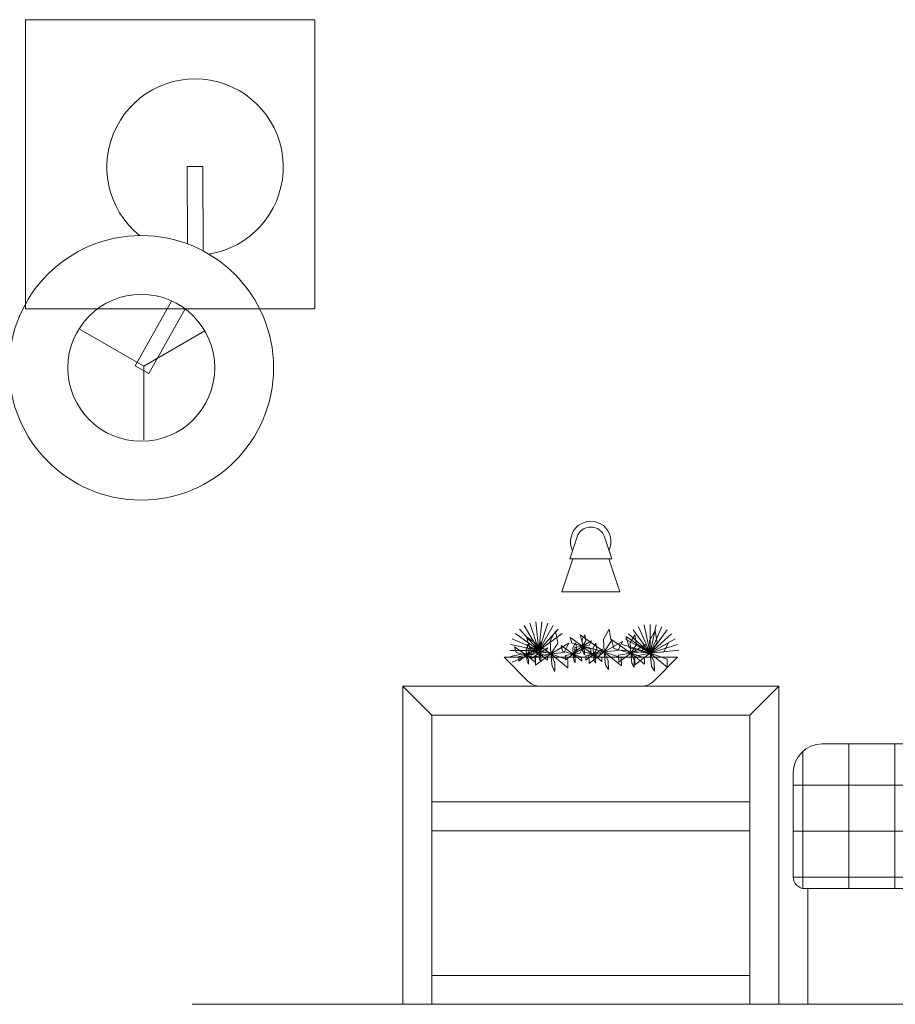
# Model space of a CAD drawing. Units: inches. Extents: x 1994 to 3075, y 3517 to 3950.
# Tile 26 of 58: x 1994.43113 to 1994.49073, y 3553.60329 to 3553.6703. Entities that reach past the tile are written whole.
import ezdxf

# ---------------------------------------------------------------- set-up
doc = ezdxf.new("R2010")
doc.units = ezdxf.units.IN
doc.layers.add('A-FURN-REFR', color=8, linetype='Continuous', lineweight=13)

msp = doc.modelspace()

# ---------------------------------------------------------------- linework, layer by layer
at = {"layer": 'A-FURN-REFR'}
for p, q in [((1994.431541370907, 3553.670297917026), (1994.431541370907, 3553.650612877656)), ((1994.451226410278, 3553.670297917026), (1994.431541370907, 3553.670297917026)), ((1994.451226410278, 3553.650612877656), (1994.451226410278, 3553.670297917026)), ((1994.442526696265, 3553.660297664388), (1994.443599002302, 3553.660302494364)), ((1994.442550361217, 3553.655043793864), (1994.442526696265, 3553.660297664388)), ((1994.443599002302, 3553.660302494364), (1994.443624860926, 3553.654561605301)), ((1994.438994690147, 3553.646750986684), (1994.441469284447, 3553.651146781573)), ((1994.431541370907, 3553.650612877656), (1994.451226410278, 3553.650612877656)), ((1994.442403711582, 3553.650620749735), (1994.439929117282, 3553.646224954846)), ((1994.439574063049, 3553.646711098967), (1994.43524393603, 3553.649211098967)), ((1994.439574063049, 3553.646711098967), (1994.443737547648, 3553.649114887921)), ((1994.439929117282, 3553.646224954846), (1994.438994690147, 3553.646750986684)), ((1994.439574063049, 3553.646711098967), (1994.439574063049, 3553.641711098967)), ((1994.468570884429, 3553.633608991265), (1994.469068334483, 3553.635101341428)), ((1994.471433271345, 3553.633608991265), (1994.470935821291, 3553.635101341428)), ((1994.46803357395, 3553.631374564225), (1994.468778382963, 3553.633608991265)), ((1994.468570884429, 3553.633608991264), (1994.471433271345, 3553.633608991265)), ((1994.471970581824, 3553.631374564225), (1994.471225772811, 3553.633608991265)), ((1994.46803357395, 3553.631374564225), (1994.471970581824, 3553.631374564225)), ((1994.465476211114, 3553.629074557141), (1994.466459409565, 3553.627369174909)), ((1994.466459409565, 3553.627369174909), (1994.465852265262, 3553.629241708899)), ((1994.46625485453, 3553.629327021937), (1994.466459409565, 3553.62736917491)), ((1994.466459409565, 3553.627369174909), (1994.466666383834, 3553.629326767666)), ((1994.46706886737, 3553.629240957197), (1994.466459409565, 3553.627369174909)), ((1994.466459409565, 3553.627369174909), (1994.467444714675, 3553.629073340861)), ((1994.473240709283, 3553.628979870546), (1994.474041371966, 3553.627181552716)), ((1994.474041371966, 3553.627181552716), (1994.473632096984, 3553.629107040119)), ((1994.474041371966, 3553.629150056654), (1994.474041371966, 3553.627181552716)), ((1994.474041371966, 3553.627181552716), (1994.474450646948, 3553.629107040119)), ((1994.474842034649, 3553.628979870546), (1994.474041371966, 3553.627181552716)), ((1994.466459409565, 3553.627369174909), (1994.464661586784, 3553.628170948567)), ((1994.464867571642, 3553.628527216263), (1994.466459409565, 3553.627369174909)), ((1994.466459409565, 3553.627369174909), (1994.465143127456, 3553.628832871995)), ((1994.46584606065, 3553.627531219063), (1994.465634292589, 3553.628302870623)), ((1994.465634292589, 3553.628302870623), (1994.467275044567, 3553.627153687641)), ((1994.467777499419, 3553.628831244294), (1994.466459409565, 3553.62736917491)), ((1994.466459409565, 3553.627369174909), (1994.468052677311, 3553.628525248281)), ((1994.467606987953, 3553.628694062704), (1994.467232384733, 3553.628020558311)), ((1994.467761039117, 3553.627872780074), (1994.467606987953, 3553.628694062704)), ((1994.468714541152, 3553.62786448459), (1994.468608657122, 3553.62825031037)), ((1994.468608657122, 3553.62825031037), (1994.469429033111, 3553.627675718879)), ((1994.469483494406, 3553.62765450469), (1994.469271726346, 3553.62842615625)), ((1994.469271726346, 3553.62842615625), (1994.470912478323, 3553.627276973268)), ((1994.469595004804, 3553.628445906411), (1994.469407703195, 3553.628109154214)), ((1994.469672030386, 3553.628035265095), (1994.469595004804, 3553.628445906411)), ((1994.471244421709, 3553.628817348331), (1994.47086981849, 3553.628143843938)), ((1994.471398472873, 3553.627996065702), (1994.471244421709, 3553.628817348331)), ((1994.472612388051, 3553.627559084138), (1994.47240061999, 3553.628330735697)), ((1994.47240061999, 3553.628330735697), (1994.474041371967, 3553.627181552715)), ((1994.472578488451, 3553.628498738949), (1994.474041371965, 3553.627181552716)), ((1994.472990738656, 3553.628432239769), (1994.47269105608, 3553.627893436255)), ((1994.474041371967, 3553.627181552716), (1994.472884314383, 3553.628774105855)), ((1994.473113979587, 3553.627775213666), (1994.472990738656, 3553.628432239769)), ((1994.474373315353, 3553.628721927778), (1994.473998712134, 3553.628048423386)), ((1994.474041371966, 3553.627181552716), (1994.475198429549, 3553.628774105855)), ((1994.475504255481, 3553.628498738949), (1994.474041371966, 3553.627181552716)), ((1994.474527366517, 3553.627900645149), (1994.474373315353, 3553.628721927778)), ((1994.464534175408, 3553.627779639515), (1994.466459409564, 3553.627369174909)), ((1994.464914215042, 3553.627238030449), (1994.464808331011, 3553.627623856228)), ((1994.464808331011, 3553.627623856228), (1994.465628707, 3553.627049264738)), ((1994.465794678693, 3553.627819452269), (1994.465607377083, 3553.627482700072)), ((1994.465753568113, 3553.627382157664), (1994.465647684083, 3553.627767983443)), ((1994.465647684083, 3553.627767983443), (1994.466468060071, 3553.627193391952)), ((1994.465871704275, 3553.627408810954), (1994.465794678693, 3553.627819452269)), ((1994.467275044567, 3553.627153687641), (1994.46584606065, 3553.627531219063)), ((1994.466634031764, 3553.627963579483), (1994.466446730155, 3553.627626827287)), ((1994.466446730155, 3553.627626827287), (1994.466468060071, 3553.627193391952)), ((1994.466468060071, 3553.627193391952), (1994.466711057347, 3553.627552938169)), ((1994.466468060071, 3553.627193391952), (1994.467088797114, 3553.627551474141)), ((1994.466711057347, 3553.627552938169), (1994.466634031764, 3553.627963579483)), ((1994.467088797114, 3553.627551474141), (1994.466930353947, 3553.62723953747)), ((1994.467232384733, 3553.628020558311), (1994.467275044567, 3553.627153687641)), ((1994.467275044567, 3553.627153687641), (1994.467761039117, 3553.627872780074)), ((1994.467275044567, 3553.627153687641), (1994.468516518652, 3553.627869852017)), ((1994.468085970577, 3553.627317511473), (1994.467980086547, 3553.627703337253)), ((1994.467980086547, 3553.627703337253), (1994.468800462536, 3553.627128745762)), ((1994.468516518652, 3553.627869852017), (1994.468199632319, 3553.627245978677)), ((1994.469429033111, 3553.627675718879), (1994.468714541152, 3553.62786448459)), ((1994.468966434229, 3553.627898933294), (1994.468779132619, 3553.627562181097)), ((1994.468779132619, 3553.627562181097), (1994.468800462536, 3553.627128745762)), ((1994.469429033111, 3553.627675718879), (1994.468909022243, 3553.627579942366)), ((1994.468909022243, 3553.627579942366), (1994.468913622717, 3553.627282713637)), ((1994.468913622717, 3553.627282713637), (1994.469429033111, 3553.627675718879)), ((1994.469043459811, 3553.627488291979), (1994.468966434229, 3553.627898933294)), ((1994.46946477712, 3553.627297252277), (1994.46935889309, 3553.627683078057)), ((1994.46935889309, 3553.627683078057), (1994.470179269078, 3553.627108486566)), ((1994.469407703195, 3553.628109154214), (1994.469429033111, 3553.627675718879)), ((1994.469429033111, 3553.627675718879), (1994.469672030386, 3553.628035265095)), ((1994.469429033111, 3553.627675718879), (1994.470049770154, 3553.628033801067)), ((1994.469891326987, 3553.627721864398), (1994.469429033111, 3553.627675718879)), ((1994.469429033111, 3553.627675718879), (1994.470007318557, 3553.627470223645)), ((1994.470013940538, 3553.62719983195), (1994.469429033111, 3553.627675718879)), ((1994.469429033111, 3553.627675718879), (1994.4695678187, 3553.627368382612)), ((1994.469477200144, 3553.627240262041), (1994.469429033111, 3553.627675718879)), ((1994.470912478323, 3553.627276973268), (1994.469483494406, 3553.62765450469)), ((1994.470049770154, 3553.628033801067), (1994.469891326987, 3553.627721864398)), ((1994.470345240772, 3553.627878674098), (1994.470157939162, 3553.627541921902)), ((1994.470157939162, 3553.627541921902), (1994.470179269078, 3553.627108486566)), ((1994.470422266354, 3553.627468032783), (1994.470345240772, 3553.627878674098)), ((1994.47086981849, 3553.628143843938), (1994.470912478323, 3553.627276973268)), ((1994.470912478323, 3553.627276973268), (1994.471398472873, 3553.627996065702)), ((1994.470912478323, 3553.627276973268), (1994.472153952409, 3553.627993137644)), ((1994.471581996814, 3553.627501964856), (1994.471412582365, 3553.628119286104)), ((1994.471412582365, 3553.628119286104), (1994.472725183947, 3553.627199939718)), ((1994.472725183947, 3553.627199939718), (1994.471581996814, 3553.627501964856)), ((1994.472153952409, 3553.627993137644), (1994.471837066075, 3553.627369264305)), ((1994.472169213469, 3553.627789853886), (1994.474041371966, 3553.627181552716)), ((1994.474041371965, 3553.627181552716), (1994.472336597549, 3553.628165804685)), ((1994.474041371967, 3553.627181552715), (1994.472612388051, 3553.627559084138)), ((1994.47269105608, 3553.627893436255), (1994.472725183947, 3553.627199939718)), ((1994.472725183947, 3553.627199939718), (1994.473113979587, 3553.627775213666)), ((1994.472725183947, 3553.627199939718), (1994.473718363215, 3553.62777287122)), ((1994.473718363215, 3553.62777287122), (1994.473464854148, 3553.627273772548)), ((1994.473998712134, 3553.628048423386), (1994.474041371967, 3553.627181552715)), ((1994.474041371966, 3553.627181552716), (1994.475746146383, 3553.628165804685)), ((1994.474041371967, 3553.627181552715), (1994.474527366517, 3553.627900645149)), ((1994.474041371967, 3553.627181552715), (1994.475282846052, 3553.627897717092)), ((1994.475913530463, 3553.627789853886), (1994.474041371966, 3553.627181552716)), ((1994.475282846052, 3553.627897717092), (1994.474965959719, 3553.627273843752)), ((1994.464096566076, 3553.626916077879), (1994.475907589698, 3553.626916077879)), ((1994.46571913314, 3553.625293510814), (1994.464096566076, 3553.626916077879)), ((1994.466459409564, 3553.627369174909), (1994.464490906004, 3553.627370391189)), ((1994.464533669651, 3553.626961089707), (1994.466459409565, 3553.62736917491)), ((1994.466459409565, 3553.62736917491), (1994.464660597373, 3553.626569623506)), ((1994.465628707, 3553.627049264738), (1994.464914215042, 3553.627238030449)), ((1994.465628707, 3553.627049264738), (1994.465108696132, 3553.626953488225)), ((1994.465108696132, 3553.626953488225), (1994.465113296607, 3553.626656259496)), ((1994.465113296607, 3553.626656259496), (1994.465628707, 3553.627049264738)), ((1994.465607377083, 3553.627482700072), (1994.465628707, 3553.627049264738)), ((1994.465628707, 3553.627049264738), (1994.465871704275, 3553.627408810954)), ((1994.465628707, 3553.627049264738), (1994.466249444043, 3553.627407346925)), ((1994.466091000876, 3553.627095410256), (1994.465628707, 3553.627049264738)), ((1994.465628707, 3553.627049264738), (1994.466206992447, 3553.626843769503)), ((1994.466213614427, 3553.626573377808), (1994.465628707, 3553.627049264738)), ((1994.465628707, 3553.627049264738), (1994.465767492589, 3553.626741928471)), ((1994.465676874034, 3553.6266138079), (1994.465628707, 3553.627049264738)), ((1994.466468060071, 3553.627193391952), (1994.465753568113, 3553.627382157664)), ((1994.466468060071, 3553.627193391952), (1994.465948049204, 3553.627097615439)), ((1994.465948049204, 3553.627097615439), (1994.465952649678, 3553.626800386711)), ((1994.465952649678, 3553.626800386711), (1994.466468060071, 3553.627193391952)), ((1994.466249444043, 3553.627407346925), (1994.466091000876, 3553.627095410256)), ((1994.466206992447, 3553.626843769503), (1994.466213614427, 3553.626573377808)), ((1994.467275044567, 3553.627153687641), (1994.466235022831, 3553.626962134615)), ((1994.466235022831, 3553.626962134615), (1994.466244223779, 3553.626367677158)), ((1994.466244223779, 3553.626367677158), (1994.467275044567, 3553.627153687641)), ((1994.466930353947, 3553.62723953747), (1994.466468060071, 3553.627193391952)), ((1994.466468060071, 3553.627193391952), (1994.467046345518, 3553.626987896718)), ((1994.467052967498, 3553.626717505024), (1994.466468060071, 3553.627193391952)), ((1994.466468060071, 3553.627193391952), (1994.46660684566, 3553.626886055686)), ((1994.466516227105, 3553.626757935114), (1994.466468060071, 3553.627193391952)), ((1994.46660684566, 3553.626886055686), (1994.46661144614, 3553.626588827035)), ((1994.467046345518, 3553.626987896718), (1994.467052967498, 3553.626717505024)), ((1994.468199632319, 3553.627245978677), (1994.467275044567, 3553.627153687641)), ((1994.467275044567, 3553.627153687641), (1994.46843161546, 3553.626742697173)), ((1994.46844485942, 3553.626201913783), (1994.467275044567, 3553.627153687641)), ((1994.467275044567, 3553.627153687641), (1994.467552615744, 3553.626539015108)), ((1994.467371378634, 3553.626282773964), (1994.467275044567, 3553.627153687641)), ((1994.468800462536, 3553.627128745762), (1994.468085970577, 3553.627317511473)), ((1994.468800462536, 3553.627128745762), (1994.468280451668, 3553.627032969249)), ((1994.468280451668, 3553.627032969249), (1994.468285052142, 3553.62673574052)), ((1994.468285052142, 3553.62673574052), (1994.468800462536, 3553.627128745762)), ((1994.468800462536, 3553.627128745762), (1994.469043459811, 3553.627488291979)), ((1994.468800462536, 3553.627128745762), (1994.469421199578, 3553.627486827951)), ((1994.469262756412, 3553.627174891281), (1994.468800462536, 3553.627128745762)), ((1994.468800462536, 3553.627128745762), (1994.469378747982, 3553.626923250528)), ((1994.469385369962, 3553.626652858833), (1994.468800462536, 3553.627128745762)), ((1994.468800462536, 3553.627128745762), (1994.468939248125, 3553.626821409495)), ((1994.468848629569, 3553.626693288924), (1994.468800462536, 3553.627128745762)), ((1994.469421199578, 3553.627486827951), (1994.469262756412, 3553.627174891281)), ((1994.469378747982, 3553.626923250528), (1994.469385369962, 3553.626652858833)), ((1994.470179269078, 3553.627108486566), (1994.46946477712, 3553.627297252277)), ((1994.46957241918, 3553.627071153961), (1994.469477200144, 3553.627240262041)), ((1994.4695678187, 3553.627368382612), (1994.46957241918, 3553.627071153961)), ((1994.470179269078, 3553.627108486566), (1994.469659258211, 3553.627012710053)), ((1994.469659258211, 3553.627012710053), (1994.469663858685, 3553.626715481325)), ((1994.469663858685, 3553.626715481325), (1994.470179269078, 3553.627108486566)), ((1994.470912478323, 3553.627276973268), (1994.469872456587, 3553.627085420242)), ((1994.469872456587, 3553.627085420242), (1994.469881657536, 3553.626490962784)), ((1994.469881657536, 3553.626490962784), (1994.470912478323, 3553.627276973268)), ((1994.470007318557, 3553.627470223645), (1994.470013940538, 3553.62719983195)), ((1994.470179269078, 3553.627108486566), (1994.470422266354, 3553.627468032783)), ((1994.470179269078, 3553.627108486566), (1994.470800006121, 3553.627466568754)), ((1994.470641562955, 3553.627154632085), (1994.470179269078, 3553.627108486566)), ((1994.470179269078, 3553.627108486566), (1994.470757554525, 3553.626902991332)), ((1994.470764176505, 3553.626632599637), (1994.470179269078, 3553.627108486566)), ((1994.470179269078, 3553.627108486566), (1994.470318054667, 3553.6268011503)), ((1994.470227436112, 3553.626673029728), (1994.470179269078, 3553.627108486566)), ((1994.470800006121, 3553.627466568754), (1994.470641562955, 3553.627154632085)), ((1994.470757554525, 3553.626902991332), (1994.470764176505, 3553.626632599637)), ((1994.471837066075, 3553.627369264305), (1994.470912478323, 3553.627276973268)), ((1994.470912478323, 3553.627276973268), (1994.472069049216, 3553.6268659828)), ((1994.472082293176, 3553.62632519941), (1994.470912478323, 3553.627276973268)), ((1994.470912478323, 3553.627276973268), (1994.471190049501, 3553.626662300735)), ((1994.47100881239, 3553.626406059591), (1994.470912478323, 3553.627276973268)), ((1994.472725183947, 3553.627199939718), (1994.471893166558, 3553.627046697297)), ((1994.471893166558, 3553.627046697297), (1994.471900527317, 3553.626571131332)), ((1994.471900527317, 3553.626571131332), (1994.472725183947, 3553.627199939718)), ((1994.472069049216, 3553.6268659828), (1994.472082293176, 3553.62632519941)), ((1994.474041371966, 3553.627181552716), (1994.472083651699, 3553.627387317408)), ((1994.473464854148, 3553.627273772548), (1994.472725183947, 3553.627199939718)), ((1994.472725183947, 3553.627199939718), (1994.473650440662, 3553.626871147343)), ((1994.473661035829, 3553.626438520633), (1994.472725183947, 3553.627199939718)), ((1994.472725183947, 3553.627199939718), (1994.472947240889, 3553.626708201692)), ((1994.4728022512, 3553.626503208778), (1994.472725183947, 3553.627199939718)), ((1994.474041371967, 3553.627181552715), (1994.473001350231, 3553.626989999689)), ((1994.473001350231, 3553.626989999689), (1994.47301055118, 3553.626395542231)), ((1994.47301055118, 3553.626395542231), (1994.474041371967, 3553.627181552715)), ((1994.473650440662, 3553.626871147343), (1994.473661035829, 3553.626438520633)), ((1994.474041371966, 3553.627181552716), (1994.475999092232, 3553.627387317408)), ((1994.474965959719, 3553.627273843752), (1994.474041371967, 3553.627181552715)), ((1994.474041371967, 3553.627181552715), (1994.47519794286, 3553.626770562247)), ((1994.47521118682, 3553.626229778858), (1994.474041371967, 3553.627181552715)), ((1994.474041371967, 3553.627181552715), (1994.474318943144, 3553.626566880183)), ((1994.474137706034, 3553.626310639039), (1994.474041371967, 3553.627181552715)), ((1994.474285022633, 3553.625293510814), (1994.475907589698, 3553.626916077879)), ((1994.465772093069, 3553.62644469982), (1994.465676874034, 3553.6266138079)), ((1994.465767492589, 3553.626741928471), (1994.465772093069, 3553.62644469982)), ((1994.46661144614, 3553.626588827035), (1994.466516227105, 3553.626757935114)), ((1994.467561816705, 3553.625944557806), (1994.467371378634, 3553.626282773964)), ((1994.467552615744, 3553.626539015108), (1994.467561816705, 3553.625944557806)), ((1994.46843161546, 3553.626742697173), (1994.46844485942, 3553.626201913783)), ((1994.468943848605, 3553.626524180844), (1994.468848629569, 3553.626693288924)), ((1994.468939248125, 3553.626821409495), (1994.468943848605, 3553.626524180844)), ((1994.470322655148, 3553.626503921649), (1994.470227436112, 3553.626673029728)), ((1994.470318054667, 3553.6268011503), (1994.470322655148, 3553.626503921649)), ((1994.471199250461, 3553.626067843433), (1994.47100881239, 3553.626406059591)), ((1994.471190049501, 3553.626662300735), (1994.471199250461, 3553.626067843433)), ((1994.472954601657, 3553.62623263585), (1994.4728022512, 3553.626503208778)), ((1994.472947240889, 3553.626708201692), (1994.472954601657, 3553.62623263585)), ((1994.474328144105, 3553.625972422881), (1994.474137706034, 3553.626310639039)), ((1994.474318943144, 3553.626566880183), (1994.474328144105, 3553.625972422881)), ((1994.47519794286, 3553.626770562247), (1994.47521118682, 3553.626229778858)), ((1994.457206802296, 3553.624947573941), (1994.457206802296, 3553.603294030634)), ((1994.457206802296, 3553.624947573942), (1994.482797353477, 3553.624947573941)), ((1994.459175306233, 3553.622979070004), (1994.457206802296, 3553.624947573941)), ((1994.46655429863, 3553.624947573942), (1994.473449857144, 3553.624947573941)), ((1994.48082884954, 3553.622979070004), (1994.482797353477, 3553.624947573941)), ((1994.482797353477, 3553.624947573941), (1994.482797353477, 3553.603294030634)), ((1994.459175306233, 3553.622979070004), (1994.48082884954, 3553.622979070004)), ((1994.459175306233, 3553.622979070004), (1994.459175306233, 3553.603294030634)), ((1994.48082884954, 3553.622979070004), (1994.48082884954, 3553.603294030634)), ((1994.485750109383, 3553.621010566067), (1994.562521762926, 3553.621010566067)), ((1994.487564222183, 3553.611168046383), (1994.487564222183, 3553.621010566067)), ((1994.490689222183, 3553.611168046383), (1994.490689222183, 3553.621010566067)), ((1994.484439222183, 3553.611178816039), (1994.484439222183, 3553.620510592858)), ((1994.483781605446, 3553.61904206213), (1994.483781605446, 3553.611955447957)), ((1994.483781605446, 3553.618198825726), (1994.564490266863, 3553.618198825726)), ((1994.459175306233, 3553.617073558193), (1994.48082884954, 3553.617073558193)), ((1994.459175306233, 3553.615105054257), (1994.48082884954, 3553.615105054257)), ((1994.483781605446, 3553.615073825726), (1994.564490266863, 3553.615073825726)), ((1994.483781633293, 3553.611948825726), (1994.564490239016, 3553.611948825726)), ((1994.48456900702, 3553.611168046383), (1994.563702865288, 3553.611168046383)), ((1994.484765857414, 3553.611168046383), (1994.484765857414, 3553.603294030634)), ((1994.459175306233, 3553.605262534571), (1994.48082884954, 3553.605262534571)), ((1994.602439621408, 3553.603294030634), (1994.442865031001, 3553.603294030634))]:
    msp.add_line(p, q, dxfattribs=at)
for radius in [0.009, 0.005]:
    msp.add_circle((1994.439410718887, 3553.646609183854), radius, dxfattribs=at)
for centre, radius, start, end in [((1994.443070972925, 3553.660269437891), 0.006, 279.0280450997825, 230.9719549002995), ((1994.470002077887, 3553.634790093627), 0.0013779527559055, 334.0196402199972, 205.9803597800028), ((1994.470002077887, 3553.634790093627), 0.0009842519685039, 18.43494882292201, 161.565051177078), ((1994.46655429863, 3553.626128676304), 0.0011811023622047, 225.0000000014038, 270.0000000003309), ((1994.473449857144, 3553.626128676304), 0.0011811023622047, 270.0000000003309, 315.000000000702), ((1994.485750109383, 3553.61904206213), 0.0019685039370079, 90, 179.9999999980146), ((1994.48456900702, 3553.611955447957), 0.0007874015748031, 179.9999999993382, 270)]:
    msp.add_arc(centre, radius, start, end, dxfattribs=at)

doc.saveas('drawing.dxf')
